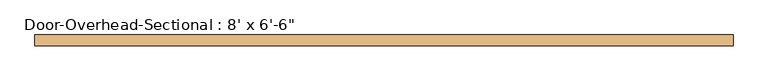
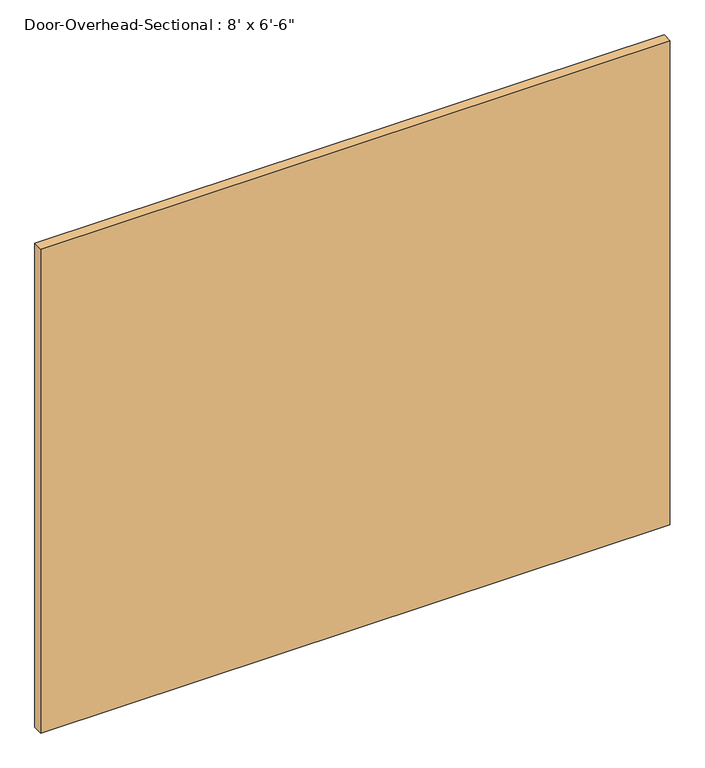
"""IFC4 building model written with IfcOpenShell, lengths in millimetres: door geometry."""

from ifc_helpers import new_model, si_unit, origin, origin_with_axes, place, context, project, spatial, polyline, outline, extrude, source, transform, mapped, element, save


def door_be48eeb6(model_context):
    return source(origin(), model_context, "Body", "SweptSolid", [
        extrude(outline(polyline([(1219.2, -101.6), (1219.2, -139.7), (-1219.2, -139.7), (-1219.2, -101.6), (1219.2, -101.6)])), origin_with_axes(), (0.0, 0.0, 1.0), 1981.2),
    ])


if __name__ == "__main__":
    model = new_model("IFC4")
    model_context = context("Model", 3, world=origin())
    ifc_project = project(units=[si_unit("LENGTHUNIT", "METRE", prefix="MILLI")], contexts=[model_context])
    site = spatial("IfcSite", under=ifc_project)
    building = spatial("IfcBuilding", under=site)
    placement = place(None, origin())
    door_shape = door_be48eeb6(model_context)
    element("IfcDoor", 1, ObjectType="Door-Overhead-Sectional : 8' x 6'-6\"", at=placement, inside=building, context=model_context, shape_type="MappedRepresentation", body=[
        mapped(door_shape, transform((0.0, 0.0, 0.0), x_axis=(1.0, 0.0, 0.0), y_axis=(0.0, 1.0, 0.0), z_axis=(0.0, 0.0, 1.0))),
    ])
    save(model, "model.ifc")

# Revit data of these elements
# Type "Door-Overhead-Sectional : 8' x 6'-6\""
#   Type Mark = "17"
#   Construction Type Id = "MDOOR"
#   Assembly Code = "B2030400"
#   Analytic Construction = "Metal"
#   Rough Width [instance default] = 8' - 0"
#   Rough Height [instance default] = 6' - 6"
#   Heat Transfer Coefficient (U) = 0.651978 BTU/(h·ft²·°F)
#   Height [instance default] = 6' - 6"
#   Thickness = 0' - 1 1/2"
#   Width [instance default] = 8' - 0"
#   Define Thermal Properties by = 1
#   Function = 1
#   Panel Material = Steel, Paint Finish, Ivory, Matte
#   Visual Light Transmittance = 0
#   Solar Heat Gain Coefficient = 0
#   Wall Closure = (empty or 0)
# Element 1 (IfcDoor, "Door-Overhead-Sectional : 8' x 6'-6\"")
#   Materials on its faces: "Steel, Paint Finish, Ivory, Matte"
# Materials
#   "Steel, Paint Finish, Ivory, Matte": class "Metal", colour RGB 247 247 239, transparency 0, Description = "Steel, paint finish, ivory, matte", Cost = 0
